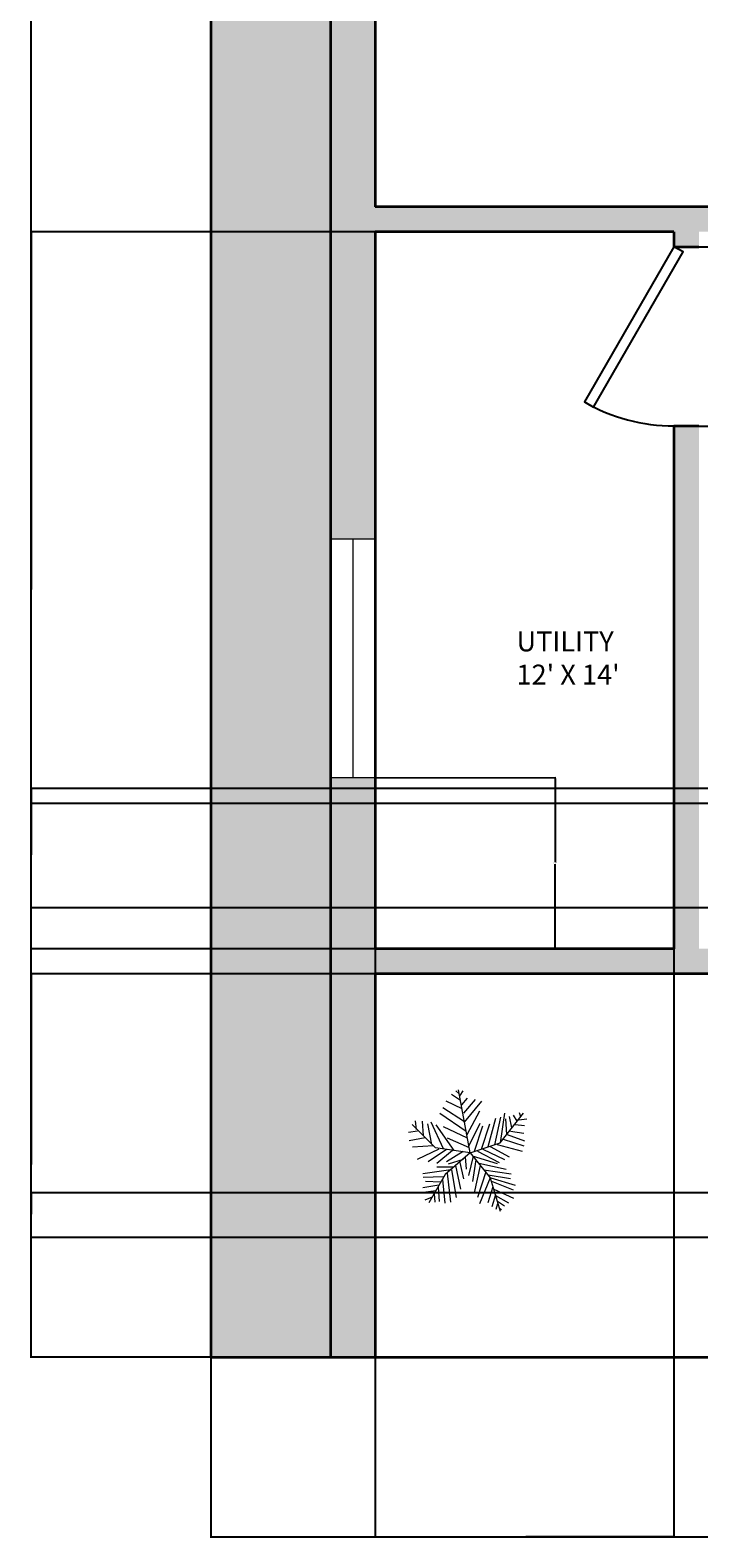
# Model space of a CAD drawing. Units: inches. Extents: x -7 to 546, y -27 to 766.
# Tile 1 of 9: x -7 to 127, y -27 to 276. Entities that reach past the tile are written whole.
import ezdxf

# ---------------------------------------------------------------- set-up
doc = ezdxf.new("R2010")
doc.units = ezdxf.units.IN
doc.header["$MEASUREMENT"] = 0
for name, color, linetype, lineweight in [('A-ANNO-DIMS', 2, 'Continuous', 18), ('A-AREA-IDEN', 7, 'Continuous', 18), ('A-WALL', 7, 'Continuous', 35), ('C-PROP', 7, 'Continuous', 35), ('doors', 40, 'Continuous', 25), ('L-PLNT', 94, 'Continuous', 18), ('window', 30, 'Continuous', 20)]:
    doc.layers.add(name, color=color, linetype=linetype, lineweight=lineweight)
doc.layers.add('A-WALL-PATT', color=251, linetype='Continuous', lineweight=13, true_color=0x636466)
doc.layers.add('L-PLNT-PATT', color=85, linetype='Continuous', lineweight=13, true_color=0x58ba48)
doc.styles.get("Standard").update_dxf_attribs({"font": 'arial.ttf'})
doc.dimstyles.get("Standard").update_dxf_attribs({"dimtxt": 0.18, "dimasz": 0.18, "dimexe": 0.18, "dimexo": 0.0625, "dimgap": 0.09, "dimtad": 0, "dimtih": 1, "dimtoh": 1, "dimdec": 4, "dimzin": 0, "dimdsep": 46, "dimtxsty": 'Standard', "dimcen": 0.09, "dimadec": 0, "dimazin": 0, "dimtfac": 1, "dimtdec": 4, "dimtofl": 0, "dimtmove": 0, "dimatfit": 3, "dimfxl": 1, "dimtolj": 1, "dimtzin": 0, "dimarcsym": 0})

# ---------------------------------------------------------------- blocks, each defined once
blk = doc.blocks.new('*U11')
for p, q in [((0, 0), (0, 100)), ((750, 0), (750, 100))]:
    blk.add_line(p, q)
blk.add_lwpolyline([(0, 0), (649.5, -375), (671.4, -337.1), (21.9, 37.9)], close=True)
blk.add_arc((0, 0), 750, 330, 0)
blk = doc.blocks.new('*U7')
for p, q in [((-10.186, 53.64), (-13.084, 55.962)), ((0, 0), (-10.5, 57)), ((-9.099, 51.782), (-6.563, 55.962)), ((-7.288, 39.707), (-21.778, 46.673)), ((-8.737, 47.138), (-17.069, 52.711)), ((-7.65, 43.423), (-2.578, 49.46)), ((-5.839, 35.992), (4.667, 48.067)), ((-5.114, 27.632), (10.463, 46.673)), ((-48.585, 21.131), (-49.309, 29.026)), ((-43.513, 28.561), (-42.427, 15.558)), ((-35.544, 28.097), (-24.314, 3.947)), ((-3.665, 19.273), (-27.574, 35.527)), ((-5.114, 28.097), (-24.676, 40.636)), ((-2.941, 16.486), (8.652, 37.85)), ((16.259, 5.805), (23.142, 31.348)), ((22.055, 7.198), (27.489, 32.277)), ((27, 9), (48, 36)), ((27.127, 9.056), (31.112, 35.992)), ((31.836, 30.883), (32.561, 16.486)), ((35.096, 32.741), (37.27, 22.524)), ((38.719, 34.134), (41.979, 28.561)), ((43.791, 29.954), (51.036, 30.883)), ((44.153, 36.456), (45.239, 32.741)), ((-47.498, 19.737), (-55.83, 18.344)), ((-40.615, 13.7), (-55.105, 10.913)), ((-31.5, 4.5), (-52.5, 25.5)), ((-38.442, 26.239), (-34.819, 7.663)), ((-14.533, 2.09), (-30.834, 25.31)), ((-24.314, 23.917), (-2.941, 13.7)), ((-20.691, 13.7), (-1.129, 4.876)), ((-1.129, 6.734), (9.014, 26.704)), ((3.942, 1.625), (11.187, 24.381)), ((10.101, 3.483), (17.708, 26.239)), ((33.285, 16.486), (48.862, 10.913)), ((36.183, 19.737), (48.137, 17.88)), ((40.53, 25.775), (48.862, 24.846)), ((-33.37, 6.269), (-52.207, 5.34)), ((-28.299, 3.483), (-47.86, -5.805)), ((-21.416, 3.018), (-38.079, -8.128)), ((0, 0), (-31.5, 4.5)), ((-15.982, 2.09), (-30.11, -9.521)), ((0, 0), (-22.5, -19.5)), ((-6.563, 1.161), (-21.416, -8.128)), ((0, 0), (27, 9)), ((0, 0), (18, -22.5)), ((6.478, 1.625), (26.04, -8.592)), ((11.187, 3.483), (30.749, -5.805)), ((18.07, 5.805), (35.096, -3.483)), ((24.229, 7.663), (46.688, 1.625)), ((29.662, 12.307), (48.137, 6.269)), ((-15.257, -12.772), (-30.11, -12.772)), ((-6.563, -5.805), (-19.967, -9.985)), ((-13.446, -11.378), (-8.737, -32.741)), ((-9.461, -8.592), (-6.201, -23.453)), ((-4.752, -3.483), (-3.665, -14.629)), ((2.493, -3.019), (-1.491, -20.202)), ((1.769, -2.555), (24.229, -9.521)), ((5.029, -6.27), (2.131, -25.775)), ((9.014, -11.378), (3.58, -35.992)), ((7.565, -9.056), (32.198, -14.629)), ((-17.431, -15.094), (-42.789, -18.809)), ((-24.314, -21.596), (-42.427, -22.06)), ((-26.849, -26.24), (-40.253, -25.775)), ((-22.5, -19.5), (-37.5, -45)), ((-25.038, -23.918), (-22.865, -45.281)), ((-20.691, -18.345), (-17.793, -44.352)), ((-17.069, -15.094), (-12.721, -40.172)), ((14.085, -16.951), (6.478, -40.172)), ((18.07, -22.524), (8.289, -45.745)), ((12.274, -15.094), (36.907, -18.809)), ((16.259, -19.738), (36.183, -22.989)), ((18, -22.5), (27, -52.5)), ((18.433, -22.524), (40.53, -29.026)), ((19.157, -25.311), (38.719, -33.206)), ((-28.299, -29.026), (-42.789, -31.348)), ((-30.834, -34.135), (-42.427, -35.528)), ((-34.457, -39.708), (-40.978, -42.494)), ((-32.646, -36.921), (-31.921, -44.352)), ((-29.023, -30.884), (-27.936, -43.887)), ((20.244, -30.419), (15.897, -44.816)), ((22.78, -37.85), (19.519, -48.532)), ((21.331, -32.741), (39.081, -40.636)), ((22.78, -38.314), (34.372, -44.816)), ((24.591, -45.745), (23.142, -50.854)), ((24.591, -43.423), (30.749, -47.603)), ((26.764, -49.925), (28.213, -50.854))]:
    blk.add_line(p, q)
blk = doc.blocks.new('WIN-48IN')
for p, q in [((0, 9), (0, 0)), ((48, 9), (0, 9)), ((0, 9), (0, 4.5)), ((48, 0), (48, 9)), ((0, 4.5), (48, 4.5)), ((0, 0), (48, 0))]:
    blk.add_line(p, q)
blk = doc.blocks.new('*D30')
at = {"layer": 'A-ANNO-DIMS', "color": 0, "lineweight": -2, "transparency": 16777216}
for p, q in [((29.23, 9.68), (29.23, -26.56)), ((509.23, 9.68), (509.23, -26.56)), ((29.41, -26.38), (268.94, -26.38)), ((509.05, -26.38), (269.52, -26.38))]:
    blk.add_line(p, q, dxfattribs=at)
at = {"layer": 'A-ANNO-DIMS', "color": 0, "transparency": 16777216}
for points in [[(29.41, -26.35), (29.41, -26.41), (29.23, -26.38)], [(509.05, -26.35), (509.05, -26.41), (509.23, -26.38)]]:
    blk.add_solid(points, dxfattribs=at)
at = {"layer": 'Defpoints', "color": 0, "transparency": 16777216}
for p in [(29.23, 9.74), (509.23, 9.74), (509.23, -26.38)]:
    blk.add_point(p, dxfattribs=at)
at = {"layer": 'A-ANNO-DIMS', "color": 0, "transparency": 16777216, "insert": (269.23, -26.38), "char_height": 0.18, "attachment_point": 5}
blk.add_mtext('\\A1;480', dxfattribs=at)
blk = doc.blocks.new('*D31')
at = {"layer": 'A-ANNO-DIMS', "color": 0, "lineweight": -2, "transparency": 16777216}
for p, q in [((29.17, 729.74), (-7.07, 729.74)), ((-6.89, 729.56), (-6.89, 369.93)), ((-6.89, 9.92), (-6.89, 369.56)), ((29.17, 9.74), (-7.07, 9.74))]:
    blk.add_line(p, q, dxfattribs=at)
at = {"layer": 'A-ANNO-DIMS', "color": 0, "transparency": 16777216}
for points in [[(-6.92, 729.56), (-6.86, 729.56), (-6.89, 729.74)], [(-6.92, 9.92), (-6.86, 9.92), (-6.89, 9.74)]]:
    blk.add_solid(points, dxfattribs=at)
at = {"layer": 'Defpoints', "color": 0, "transparency": 16777216}
for p in [(-6.89, 729.74), (29.23, 729.74), (29.23, 9.74)]:
    blk.add_point(p, dxfattribs=at)
at = {"layer": 'A-ANNO-DIMS', "color": 0, "transparency": 16777216, "insert": (-6.89, 369.74), "char_height": 0.18, "attachment_point": 5}
blk.add_mtext('\\A1;720', dxfattribs=at)
blk = doc.blocks.new('*D48')
at = {"layer": 'A-ANNO-DIMS', "color": 0, "lineweight": -2, "transparency": 16777216}
for p, q in [((62.23, 91.68), (62.23, -26.56)), ((122.23, 91.68), (122.23, -26.56)), ((62.41, -26.38), (92.01, -26.38)), ((122.05, -26.38), (92.45, -26.38))]:
    blk.add_line(p, q, dxfattribs=at)
at = {"layer": 'A-ANNO-DIMS', "color": 0, "transparency": 16777216}
for points in [[(62.41, -26.35), (62.41, -26.41), (62.23, -26.38)], [(122.05, -26.35), (122.05, -26.41), (122.23, -26.38)]]:
    blk.add_solid(points, dxfattribs=at)
at = {"layer": 'Defpoints', "color": 0, "transparency": 16777216}
for p in [(62.23, 91.74), (122.23, 91.74), (122.23, -26.38)]:
    blk.add_point(p, dxfattribs=at)
at = {"layer": 'A-ANNO-DIMS', "color": 0, "transparency": 16777216, "insert": (92.23, -26.38), "char_height": 0.18, "attachment_point": 5}
blk.add_mtext('\\A1;60', dxfattribs=at)
blk = doc.blocks.new('*D50')
at = {"layer": 'A-ANNO-DIMS', "color": 0, "lineweight": -2, "transparency": 16777216}
for p, q in [((62.17, 235.74), (-7.07, 235.74)), ((-6.89, 235.56), (-6.89, 163.92)), ((-6.89, 91.92), (-6.89, 163.56)), ((62.17, 91.74), (-7.07, 91.74))]:
    blk.add_line(p, q, dxfattribs=at)
at = {"layer": 'A-ANNO-DIMS', "color": 0, "transparency": 16777216}
for points in [[(-6.92, 235.56), (-6.86, 235.56), (-6.89, 235.74)], [(-6.92, 91.92), (-6.86, 91.92), (-6.89, 91.74)]]:
    blk.add_solid(points, dxfattribs=at)
at = {"layer": 'Defpoints', "color": 0, "transparency": 16777216}
for p in [(-6.89, 235.74), (62.23, 235.74), (62.23, 91.74)]:
    blk.add_point(p, dxfattribs=at)
at = {"layer": 'A-ANNO-DIMS', "color": 0, "transparency": 16777216, "insert": (-6.89, 163.74), "char_height": 0.18, "attachment_point": 5}
blk.add_mtext('\\A1;144', dxfattribs=at)
blk = doc.blocks.new('*D52')
at = {"layer": 'A-ANNO-DIMS', "color": 0, "lineweight": -2, "transparency": 16777216}
for p, q in [((122.29, 232.74), (158.54, 232.74)), ((158.36, 232.56), (158.36, 214.93)), ((158.36, 196.92), (158.36, 214.56)), ((122.29, 196.74), (158.54, 196.74))]:
    blk.add_line(p, q, dxfattribs=at)
at = {"layer": 'A-ANNO-DIMS', "color": 0, "transparency": 16777216}
for points in [[(158.33, 232.56), (158.39, 232.56), (158.36, 232.74)], [(158.33, 196.92), (158.39, 196.92), (158.36, 196.74)]]:
    blk.add_solid(points, dxfattribs=at)
at = {"layer": 'Defpoints', "color": 0, "transparency": 16777216}
for p in [(122.23, 232.74), (122.23, 196.74), (158.36, 196.74)]:
    blk.add_point(p, dxfattribs=at)
at = {"layer": 'A-ANNO-DIMS', "color": 0, "transparency": 16777216, "insert": (158.36, 214.74), "char_height": 0.18, "attachment_point": 5}
blk.add_mtext('\\A1;36', dxfattribs=at)
blk = doc.blocks.new('*D54')
at = {"layer": 'A-ANNO-DIMS', "color": 0, "lineweight": -2, "transparency": 16777216}
for p, q in [((229.86, 123.94), (-7.07, 123.94)), ((-6.89, 123.76), (-6.89, 112.12)), ((-6.89, 100.12), (-6.89, 111.76)), ((229.86, 99.94), (-7.07, 99.94))]:
    blk.add_line(p, q, dxfattribs=at)
at = {"layer": 'A-ANNO-DIMS', "color": 0, "transparency": 16777216}
for points in [[(-6.92, 123.76), (-6.86, 123.76), (-6.89, 123.94)], [(-6.92, 100.12), (-6.86, 100.12), (-6.89, 99.94)]]:
    blk.add_solid(points, dxfattribs=at)
at = {"layer": 'Defpoints', "color": 0, "transparency": 16777216}
for p in [(229.93, 123.94), (-6.89, 99.94), (229.93, 99.94)]:
    blk.add_point(p, dxfattribs=at)
at = {"layer": 'A-ANNO-DIMS', "color": 0, "transparency": 16777216, "insert": (-6.89, 111.94), "char_height": 0.18, "attachment_point": 5}
blk.add_mtext('\\A1;24', dxfattribs=at)
blk = doc.blocks.new('*D62')
at = {"layer": 'A-ANNO-DIMS', "color": 0, "lineweight": -2, "transparency": 16777216}
for p, q in [((62.29, 126.11), (98.53, 126.12)), ((98.35, 125.94), (98.35, 109.12)), ((98.36, 91.93), (98.35, 108.75)), ((62.29, 91.74), (98.54, 91.75))]:
    blk.add_line(p, q, dxfattribs=at)
at = {"layer": 'A-ANNO-DIMS', "color": 0, "transparency": 16777216}
for points in [[(98.38, 125.94), (98.32, 125.94), (98.35, 126.12)], [(98.39, 91.93), (98.33, 91.93), (98.36, 91.75)]]:
    blk.add_solid(points, dxfattribs=at)
at = {"layer": 'Defpoints', "color": 0, "transparency": 16777216}
for p in [(62.23, 126.11), (62.23, 91.74), (98.36, 91.75)]:
    blk.add_point(p, dxfattribs=at)
at = {"layer": 'A-ANNO-DIMS', "color": 0, "transparency": 16777216, "insert": (98.35, 108.93), "char_height": 0.18, "attachment_point": 5}
blk.add_mtext('\\A1;34.37', dxfattribs=at)
blk = doc.blocks.new('*D65')
at = {"layer": 'A-ANNO-DIMS', "color": 0, "lineweight": -2, "transparency": 16777216}
for p, q in [((461.17, 42.74), (-7.07, 42.74)), ((-6.89, 42.56), (-6.89, 38.43)), ((-6.89, 33.92), (-6.89, 38.06)), ((461.17, 33.74), (-7.07, 33.74))]:
    blk.add_line(p, q, dxfattribs=at)
at = {"layer": 'A-ANNO-DIMS', "color": 0, "transparency": 16777216}
for points in [[(-6.92, 42.56), (-6.86, 42.56), (-6.89, 42.74)], [(-6.92, 33.92), (-6.86, 33.92), (-6.89, 33.74)]]:
    blk.add_solid(points, dxfattribs=at)
at = {"layer": 'Defpoints', "color": 0, "transparency": 16777216}
for p in [(-6.89, 42.74), (461.23, 42.74), (461.23, 33.74)]:
    blk.add_point(p, dxfattribs=at)
at = {"layer": 'A-ANNO-DIMS', "color": 0, "transparency": 16777216, "insert": (-6.89, 38.24), "char_height": 0.18, "attachment_point": 5}
blk.add_mtext('\\A1;9', dxfattribs=at)
blk = doc.blocks.new('*D69')
at = {"layer": 'A-ANNO-DIMS', "color": 0, "lineweight": -2, "transparency": 16777216}
for p, q in [((167.36, 120.94), (-7.07, 120.94)), ((-6.89, 120.76), (-6.89, 110.62)), ((-6.89, 100.12), (-6.89, 110.26)), ((167.36, 99.94), (-7.07, 99.94))]:
    blk.add_line(p, q, dxfattribs=at)
at = {"layer": 'A-ANNO-DIMS', "color": 0, "transparency": 16777216}
for points in [[(-6.92, 120.76), (-6.86, 120.76), (-6.89, 120.94)], [(-6.92, 100.12), (-6.86, 100.12), (-6.89, 99.94)]]:
    blk.add_solid(points, dxfattribs=at)
at = {"layer": 'Defpoints', "color": 0, "transparency": 16777216}
for p in [(-6.89, 120.94), (167.43, 120.94), (167.43, 99.94)]:
    blk.add_point(p, dxfattribs=at)
at = {"layer": 'A-ANNO-DIMS', "color": 0, "transparency": 16777216, "insert": (-6.89, 110.44), "char_height": 0.18, "attachment_point": 5}
blk.add_mtext('\\A1;21', dxfattribs=at)
blk = doc.blocks.new('*D79')
at = {"layer": 'A-ANNO-DIMS', "color": 0, "lineweight": -2, "transparency": 16777216}
for p, q in [((62.169415, 86.743976), (-7.073085, 86.743976)), ((-6.893085, 86.563976), (-6.893085, 48.423976)), ((-6.893085, 9.923976), (-6.893085, 48.063976)), ((62.169415, 9.743976), (-7.073085, 9.743976))]:
    blk.add_line(p, q, dxfattribs=at)
at = {"layer": 'A-ANNO-DIMS', "color": 0, "transparency": 16777216}
for points in [[(-6.923085, 86.563976), (-6.863085, 86.563976), (-6.893085, 86.743976)], [(-6.923085, 9.923976), (-6.863085, 9.923976), (-6.893085, 9.743976)]]:
    blk.add_solid(points, dxfattribs=at)
at = {"layer": 'Defpoints', "color": 0, "transparency": 16777216}
for p in [(62.231915, 86.743976), (-6.893085, 9.743976), (62.231915, 9.743976)]:
    blk.add_point(p, dxfattribs=at)
at = {"layer": 'A-ANNO-DIMS', "color": 0, "transparency": 16777216, "insert": (-6.893085, 48.243976), "char_height": 0.18, "attachment_point": 5}
blk.add_mtext('\\A1;77', dxfattribs=at)
blk = doc.blocks.new('*D81')
at = {"layer": 'A-ANNO-DIMS', "color": 0, "lineweight": -2, "transparency": 16777216}
for p, q in [((62.23, 240.81), (62.23, 766.05)), ((62.41, 765.87), (194.44, 765.87)), ((327.05, 765.87), (195.02, 765.87)), ((327.23, 234.81), (327.23, 766.05))]:
    blk.add_line(p, q, dxfattribs=at)
at = {"layer": 'A-ANNO-DIMS', "color": 0, "transparency": 16777216}
for points in [[(62.41, 765.9), (62.41, 765.84), (62.23, 765.87)], [(327.05, 765.9), (327.05, 765.84), (327.23, 765.87)]]:
    blk.add_solid(points, dxfattribs=at)
at = {"layer": 'Defpoints', "color": 0, "transparency": 16777216}
for p in [(327.23, 765.87), (62.23, 240.74), (327.23, 234.74)]:
    blk.add_point(p, dxfattribs=at)
at = {"layer": 'A-ANNO-DIMS', "color": 0, "transparency": 16777216, "insert": (194.73, 765.87), "char_height": 0.18, "attachment_point": 5}
blk.add_mtext('\\A1;265', dxfattribs=at)

msp = doc.modelspace()

# ---------------------------------------------------------------- hatches: boundary and pattern name
at = {"layer": 'A-WALL-PATT'}
h = msp.add_hatch(color=256, dxfattribs=at)
h.dxf.hatch_style = 1
h.paths.add_polyline_path([(62.2319, 696.744), (86.6896, 696.744), (86.6896, 705.744), (53.2319, 705.744), (53.2319, 627.8642), (57.7271, 627.8642), (62.2319, 627.8642)])
h.paths.add_polyline_path([(229.7414, 705.744), (134.6896, 705.744), (134.6896, 696.744), (206.2319, 696.744), (206.2319, 567.744), (211.2319, 567.744), (211.2319, 595.744), (214.2319, 595.744), (214.2319, 600.744), (211.2319, 600.744), (211.2319, 696.744), (229.7414, 696.744)])
h.paths.add_polyline_path([(293.8423, 705.744), (253.7414, 705.744), (253.7414, 696.744), (274.2319, 696.744), (274.2319, 600.744), (279.2319, 600.744), (279.2319, 696.744), (293.8423, 696.744)])
h.paths.add_polyline_path([(393.9743, 705.744), (317.8423, 705.744), (317.8423, 696.744), (327.2319, 696.744), (327.2319, 651.744), (332.2319, 651.744), (332.2319, 696.744), (393.9743, 696.744)])
h.paths.add_polyline_path([(485.2319, 705.744), (441.9743, 705.744), (441.9743, 696.744), (476.2319, 696.744), (476.2319, 663.6898), (480.7319, 663.6898), (485.2319, 663.6898)])
h.paths.add_polyline_path([(485.2319, 615.6898), (476.2319, 615.6898), (476.2319, 528.744), (332.2319, 528.744), (332.2319, 531.744), (327.2319, 531.744), (327.2319, 523.744), (375.2319, 523.744), (375.2319, 427.744), (327.2319, 427.744), (327.2319, 419.744), (332.2319, 419.744), (332.2319, 422.744), (413.089, 422.744), (413.089, 427.744), (380.2319, 427.744), (380.2319, 523.744), (476.2319, 523.744), (476.2319, 490.9334), (485.2319, 490.9334)])
h.paths.add_polyline_path([(485.2319, 466.9334), (476.2319, 466.9334), (476.2319, 370.0932), (480.7319, 370.0932), (485.2319, 370.0932)])
h.paths.add_polyline_path([(485.2319, 322.0932), (476.2319, 322.0932), (476.2319, 278.744), (332.2319, 278.744), (332.2319, 383.744), (327.2319, 383.744), (327.2319, 273.744), (327.2319, 270.744), (332.2319, 270.744), (332.2319, 273.744), (476.2319, 273.744), (476.2319, 201.0338), (480.7319, 201.0338), (485.2319, 201.0338)])
h.paths.add_polyline_path([(485.2319, 153.0338), (476.2319, 153.0338), (476.2319, 42.744), (461.2319, 42.744), (461.2319, 33.744), (485.2319, 33.744)])
h.paths.add_polyline_path([(332.2319, 234.744), (327.2319, 234.744), (327.2319, 160.744), (315.2319, 160.744), (315.2319, 151.744), (327.2319, 151.744), (327.2319, 33.744), (332.2319, 33.744)])
h.paths.add_polyline_path([(252.2319, 151.744), (258.4464, 151.744), (264.2319, 151.744), (264.2319, 160.744), (252.2319, 160.744), (252.2319, 172.744), (247.2319, 172.744), (247.2319, 91.744), (127.2319, 91.744), (127.2319, 196.744), (122.2319, 196.744), (122.2319, 91.744), (62.2319, 91.744), (62.2319, 126.1124), (53.2319, 126.1124), (53.2319, 9.744), (62.2319, 9.744), (62.2319, 86.744), (247.2319, 86.744), (247.2319, 33.744), (252.2319, 33.744), (252.2319, 53.744)])
h.paths.add_polyline_path([(62.2319, 235.744), (122.2319, 235.744), (122.2319, 232.744), (127.2319, 232.744), (127.2319, 235.744), (247.2319, 235.744), (247.2319, 220.744), (252.2319, 220.744), (252.2319, 240.744), (250.6678, 240.744), (247.2319, 240.744), (62.2319, 240.744), (62.2319, 322.0932), (53.2319, 322.0932), (53.2319, 174.1124), (57.7271, 174.1124), (62.2319, 174.1124)])
at = {"layer": 'L-PLNT-PATT'}
h = msp.add_hatch(color=256, dxfattribs=at)
h.dxf.hatch_style = 1
h.paths.add_polyline_path([(509.2319, 729.744), (29.2319, 729.744), (29.2319, 9.744), (53.2319, 9.744), (53.2319, 705.744), (485.2319, 705.744), (485.2319, 33.744), (461.2319, 33.744), (461.2319, 9.744), (509.2319, 9.744)])

# ---------------------------------------------------------------- linework, layer by layer
at = {"layer": 'A-WALL'}
for p, q in [((62.2319, 523.744), (62.2319, 240.744)), ((247.2319, 240.744), (62.2319, 240.744)), ((122.2319, 235.744), (62.2319, 235.744)), ((62.2319, 235.744), (62.2319, 91.744)), ((122.2319, 235.744), (122.2319, 232.744)), ((122.2319, 235.744), (122.2319, 232.744)), ((122.2319, 232.744), (127.2319, 232.744)), ((122.2319, 196.744), (122.2319, 91.744)), ((122.2319, 196.744), (127.2319, 196.744)), ((122.2319, 91.744), (62.2319, 91.744)), ((247.2319, 86.744), (62.2319, 86.744)), ((62.2319, 86.744), (62.2319, 9.744))]:
    msp.add_line(p, q, dxfattribs=at)
msp.add_lwpolyline([(461.2319, 33.744), (485.2319, 33.744), (485.2319, 705.744), (53.2319, 705.744), (53.2319, 9.744)], dxfattribs=at)
at = {"layer": 'C-PROP'}
msp.add_lwpolyline([(29.2319, 9.744), (509.2319, 9.744), (509.2319, 729.744), (29.2319, 729.744)], close=True, dxfattribs=at)

# ---------------------------------------------------------------- block references
at = {"layer": 'doors', "xscale": 0.0480000000000013, "yscale": 0.0480000000000013, "zscale": 0.0480000000000013, "rotation": 270.0000000000029}
msp.add_blockref('*U11', (122.2319, 232.744), dxfattribs=at)
at = {"layer": 'L-PLNT', "xscale": 0.2228533388545292, "yscale": 0.2228533388545292, "zscale": 0.2228533388545292}
msp.add_blockref('*U7', (81.3169, 50.7409), dxfattribs=at)
at = {"layer": 'window', "extrusion": (0, 0, -1), "zscale": -1, "rotation": 270.0000000000001}
msp.add_blockref('WIN-48IN', (-62.227, 174.112), dxfattribs=at)

# ---------------------------------------------------------------- texts
at = {"layer": 'A-AREA-IDEN', "insert": (89.38, 155.483), "char_height": 4, "attachment_point": 1}
msp.add_mtext_dynamic_manual_height_columns(" UTILITY\\P 12' X 14'", width=80.777321, gutter_width=1, heights=[0], dxfattribs=at)

# ---------------------------------------------------------------- dimensions: what is measured, and where the dimension line sits
at = {"layer": 'A-ANNO-DIMS'}
for base, p1, p2, picture, middle in [((327.2319, 765.869), (62.2319, 240.744), (327.2319, 234.744), '*D81', (194.7319, 765.869)), ((122.2319, -26.381), (62.2319, 91.744), (122.2319, 91.744), '*D48', (92.2319, -26.381)), ((509.2319, -26.381), (29.2319, 9.744), (509.2319, 9.744), '*D30', (269.2319, -26.381))]:
    dim = msp.add_linear_dim(base=base, p1=p1, p2=p2, dimstyle='Standard', override={"dimdec": 0, "dimlfac": 1, "dimrnd": 0, "dimzin": 0, "dimdsep": 46, "dimlunit": 2}, dxfattribs=at)
    dim.commit()
    dim.dimension.update_dxf_attribs({"geometry": picture, "text_midpoint": middle})
for base, p1, p2, angle, override, picture, middle in [((-6.8931, 729.744), (29.2319, 9.744), (29.2319, 729.744), 90, {"dimdec": 0, "dimlfac": 1, "dimrnd": 0, "dimzin": 0, "dimdsep": 46, "dimlunit": 2}, '*D31', (-6.8931, 369.744)), ((-6.8931, 235.744), (62.2319, 91.744), (62.2319, 235.744), 90, {"dimdec": 0, "dimlfac": 1, "dimrnd": 0, "dimzin": 0, "dimdsep": 46, "dimlunit": 2}, '*D50', (-6.8931, 163.744)), ((158.3569, 196.744), (122.2319, 232.744), (122.2319, 196.744), 270, {"dimdec": 0, "dimlfac": 1, "dimrnd": 0, "dimzin": 0, "dimdsep": 46, "dimlunit": 2}, '*D52', (158.3569, 214.744)), ((98.3569, 91.7491), (62.2271, 126.1124), (62.2319, 91.744), 270.008094, {"dimdec": 2, "dimlfac": 1, "dimrnd": 0, "dimzin": 0, "dimdsep": 46, "dimlunit": 2}, '*D62', (98.3545, 108.9333)), ((-6.8931, 99.9426), (229.9271, 123.9426), (229.9271, 99.9426), 90, {"dimdec": 0, "dimlfac": 1, "dimrnd": 0, "dimzin": 0, "dimdsep": 46, "dimlunit": 2}, '*D54', (-6.8931, 111.9426)), ((-6.8931, 120.9426), (167.4271, 99.9426), (167.4271, 120.9426), 90, {"dimdec": 0, "dimlfac": 1, "dimrnd": 0, "dimzin": 0, "dimdsep": 46, "dimlunit": 2}, '*D69', (-6.8931, 110.4426)), ((-6.8931, 9.744), (62.2319, 86.744), (62.2319, 9.744), 90, {"dimdec": 0, "dimlfac": 1, "dimrnd": 0, "dimzin": 0, "dimdsep": 46, "dimlunit": 2}, '*D79', (-6.8931, 48.244)), ((-6.8931, 42.744), (461.2319, 33.744), (461.2319, 42.744), 90, {"dimdec": 0, "dimlfac": 1, "dimrnd": 0, "dimzin": 0, "dimdsep": 46, "dimlunit": 2}, '*D65', (-6.8931, 38.244))]:
    dim = msp.add_linear_dim(base=base, p1=p1, p2=p2, angle=angle, dimstyle='Standard', override=override, dxfattribs=at)
    dim.commit()
    dim.dimension.update_dxf_attribs({"geometry": picture, "text_midpoint": middle})

doc.saveas('drawing.dxf')
